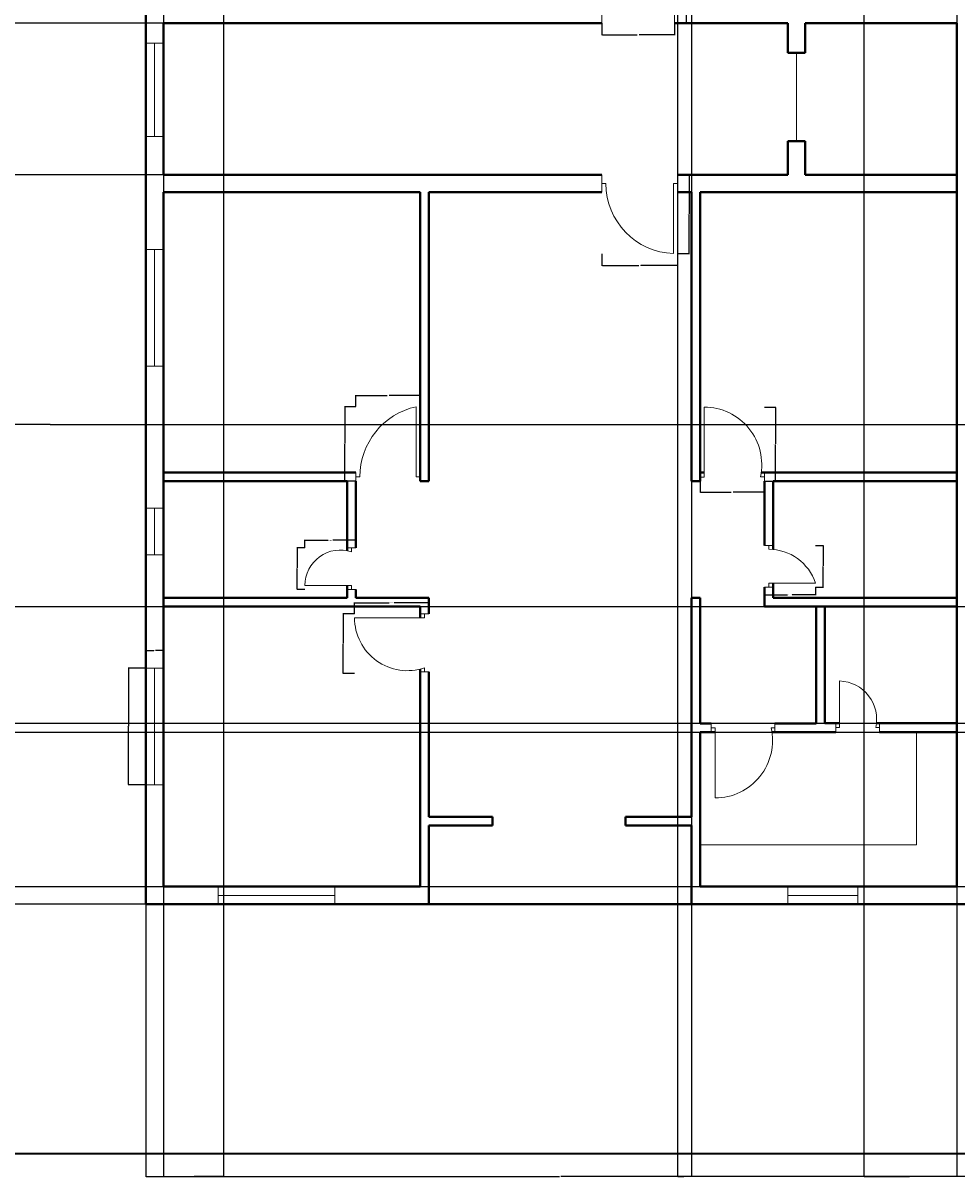
# Model space of a CAD drawing. Units: inches. Extents: x 1355 to 2746, y 1171 to 2751.
# Tile 14 of 24: x 2017 to 2497, y 1171 to 1764. Entities that reach past the tile are written whole.
import ezdxf

# ---------------------------------------------------------------- set-up
doc = ezdxf.new("R2010")
doc.units = ezdxf.units.IN
for name, color, linetype, lineweight in [('A-ANNO-DIMS', 2, 'Continuous', 18), ('A-ANNO-SYMB', 2, 'Continuous', 25), ('A-ANNO-TTLB', 7, 'Continuous', 35), ('A-DOOR', 3, 'Continuous', 20), ('A-FLOR-CASE', 30, 'Continuous', 20), ('A-GLAZ', 4, 'Continuous', 18), ('A-WALL', 7, 'Continuous', 40)]:
    doc.layers.add(name, color=color, linetype=linetype, lineweight=lineweight)
doc.styles.get("Standard").update_dxf_attribs({"font": 'arial.ttf'})
doc.dimstyles.get("Standard").update_dxf_attribs({"dimtxt": 0.18, "dimasz": 0.18, "dimexe": 0.18, "dimexo": 0.0625, "dimgap": 0.09, "dimtad": 0, "dimtih": 1, "dimtoh": 1, "dimdec": 4, "dimzin": 0, "dimdsep": 46, "dimtxsty": 'Standard', "dimcen": 0.09, "dimadec": 0, "dimazin": 0, "dimtfac": 1, "dimtdec": 4, "dimtofl": 0, "dimtmove": 0, "dimatfit": 3, "dimfxl": 1, "dimtolj": 1, "dimtzin": 0, "dimarcsym": 0})

# ---------------------------------------------------------------- blocks, each defined once
blk = doc.blocks.new('WINDOW-PLAN-24')
for p, q in [((0, 24), (9, 24)), ((9, 24), (4.5, 24)), ((4.5, 24), (4.5, 0)), ((4.5, 0), (0, 0)), ((0, 0), (9, 0))]:
    blk.add_line(p, q)
blk = doc.blocks.new('WINDOW-PLAN-60')
for p, q in [((0, 60), (9, 60)), ((9, 60), (4.5, 60)), ((4.5, 60), (4.5, 0)), ((4.5, 0), (0, 0)), ((0, 0), (9, 0))]:
    blk.add_line(p, q)
blk = doc.blocks.new('WINDOW-PLAN-60-2')
for p, q in [((4.5, 60), (0, 60)), ((0, 60), (9, 60)), ((4.5, 0), (4.5, 60)), ((9, 0), (0, 0)), ((0, 0), (4.5, 0))]:
    blk.add_line(p, q)
blk = doc.blocks.new('WINDOW-PLAN-36')
for p, q in [((0, 9), (0, 0)), ((36, 4.5), (36, 9)), ((36, 9), (36, 0)), ((0, 0), (0, 4.5)), ((0, 4.5), (36, 4.5))]:
    blk.add_line(p, q)
blk = doc.blocks.new('WINDOW-PLAN-48')
for p, q in [((9, 48), (0, 48)), ((0, 48), (4.5, 48)), ((4.5, 48), (4.5, 12)), ((4.5, 12), (4.5, 0)), ((4.5, 0), (0, 0)), ((0, 0), (9, 0))]:
    blk.add_line(p, q)
blk = doc.blocks.new('DOOR-ENTRY-N')
for p, q in [((35.29, 4.5), (35.29, 40.5)), ((0, 9), (0, 0)), ((37.29, 9), (37.29, 0)), ((0, 0), (0, 4.5)), ((0, 4.5), (2, 4.5)), ((37.29, 4.5), (35.29, 4.5)), ((37.29, 0), (37.29, 4.5))]:
    blk.add_line(p, q)
blk.add_arc((38.11, 4.5), 36.11, 94.47163, 180)
blk = doc.blocks.new('DOOR-BED-SE')
for p, q in [((2, 2.1), (2, 38.1)), ((0, 2.1), (2, 2.1)), ((33, 2.25), (31, 2.25)), ((33, 0), (33, 4.5)), ((33, 4.5), (33, 2.25))]:
    blk.add_line(p, q)
blk.add_arc((2, 8.44), 29.65, 347.94805, 90)
blk = doc.blocks.new('DOOR-WC-SE')
for p, q in [((0, 21.41), (4.5, 21.41)), ((4.5, 21.41), (2.25, 21.41)), ((2.25, 21.41), (2.25, 19.41)), ((2.25, 0), (2.25, 2)), ((2.25, 2), (26.25, 2)), ((4.5, 0), (0, 0)), ((0, 0), (2.25, 0))]:
    blk.add_line(p, q)
blk.add_arc((2.25, -5.83), 25.25, 18.07862, 90)
blk = doc.blocks.new('DOOR-BED-SW')
for p, q in [((31, 2.25), (31, 38.25)), ((0, 0), (0, 4.5)), ((0, 2.25), (2, 2.25)), ((33, 2.25), (31, 2.25))]:
    blk.add_line(p, q)
blk.add_arc((38.85, 2.25), 36.84, 102.29325, 180)
blk = doc.blocks.new('DOOR-WC-SW')
for p, q in [((21.75, 21.26), (26.25, 21.26)), ((26.25, 21.26), (24, 21.26)), ((24, 21.26), (24, 19.26)), ((24, 2), (0, 2)), ((24, 0), (24, 2)), ((26.25, 0), (21.75, 0)), ((21.75, 0), (24, 0))]:
    blk.add_line(p, q)
blk.add_arc((18.21, 2), 18.21, 71.45684, 180)
blk = doc.blocks.new('DOOR-BEDROOM-SW')
for p, q in [((33.75, 29.78), (38.25, 29.78)), ((38.25, 29.78), (36, 29.78)), ((36, 29.78), (36, 27.78)), ((36, 27.78), (0, 27.78)), ((33.75, 0), (38.25, 0)), ((36, 0), (36, 2)), ((38.25, 0), (36, 0))]:
    blk.add_line(p, q)
blk.add_arc((27.23, 27.78), 27.23, 180, 288.79179)
blk = doc.blocks.new('DOOR-UTILITY-S')
for p, q in [((2, 2.25), (2, 26.25)), ((0, 4.5), (0, 0)), ((0, 0), (0, 2.25)), ((0, 2.25), (2, 2.25)), ((22.55, 2.25), (20.55, 2.25)), ((22.55, 4.5), (22.55, 0)), ((22.55, 0), (22.55, 2.25))]:
    blk.add_line(p, q)
blk.add_arc((1.26, 6.51), 19.76, 347.56133, 87.85632)
blk = doc.blocks.new('DOOR-KITCHEN-S')
for p, q in [((0, 38.25), (0, 33.75)), ((0, 33.75), (0, 36)), ((0, 36), (2, 36)), ((2, 36), (2, 0)), ((32.75, 36), (30.75, 36)), ((32.75, 38.25), (32.75, 33.89)), ((32.75, 33.89), (32.75, 36))]:
    blk.add_line(p, q)
blk.add_arc((2, 29.48), 29.48, 270, 12.78512)
blk = doc.blocks.new('DOOR-ENTRY-S')
for p, q in [((0, 40.5), (0, 31.5)), ((0, 36), (2, 36)), ((38.81, 36), (36.81, 36)), ((36.81, 36), (36.81, 0)), ((38.81, 31.5), (38.81, 40.5))]:
    blk.add_line(p, q)
blk.add_arc((38.02, 36), 36.02, 180, 268.07058)
blk = doc.blocks.new('*D47')
at = {"layer": 'A-ANNO-DIMS', "color": 0, "lineweight": -2, "transparency": 16777216}
for p, q in [((2080.33, 1432.65), (2071.21, 1432.65)), ((2071.39, 1432.47), (2071.39, 1402.84)), ((2071.39, 1372.83), (2071.39, 1402.47)), ((2080.33, 1372.65), (2071.21, 1372.65))]:
    blk.add_line(p, q, dxfattribs=at)
at = {"layer": 'A-ANNO-DIMS', "color": 0, "transparency": 16777216}
for points in [[(2071.36, 1432.47), (2071.42, 1432.47), (2071.39, 1432.65)], [(2071.36, 1372.83), (2071.42, 1372.83), (2071.39, 1372.65)]]:
    blk.add_solid(points, dxfattribs=at)
at = {"layer": 'Defpoints', "color": 0, "transparency": 16777216}
for p in [(2071.39, 1432.65), (2080.39, 1432.65), (2080.39, 1372.65)]:
    blk.add_point(p, dxfattribs=at)
at = {"layer": 'A-ANNO-DIMS', "color": 0, "transparency": 16777216, "insert": (2071.39, 1402.65), "char_height": 0.18, "attachment_point": 5}
blk.add_mtext('\\A1;WINDOW 60 TYP.', dxfattribs=at)
blk = doc.blocks.new('*D48')
at = {"layer": 'A-ANNO-DIMS', "color": 0, "lineweight": -2, "transparency": 16777216}
for p, q in [((2080.39, 1432.72), (2080.39, 1441.83)), ((2080.57, 1441.65), (2084.43, 1441.65)), ((2089.21, 1441.65), (2085.35, 1441.65)), ((2089.39, 1432.72), (2089.39, 1441.83))]:
    blk.add_line(p, q, dxfattribs=at)
at = {"layer": 'A-ANNO-DIMS', "color": 0, "transparency": 16777216}
for points in [[(2080.57, 1441.68), (2080.57, 1441.62), (2080.39, 1441.65)], [(2089.21, 1441.68), (2089.21, 1441.62), (2089.39, 1441.65)]]:
    blk.add_solid(points, dxfattribs=at)
at = {"layer": 'Defpoints', "color": 0, "transparency": 16777216}
for p in [(2089.39, 1441.65), (2080.39, 1432.65), (2089.39, 1432.65)]:
    blk.add_point(p, dxfattribs=at)
at = {"layer": 'A-ANNO-DIMS', "color": 0, "transparency": 16777216, "insert": (2084.89, 1441.65), "char_height": 0.18, "attachment_point": 5}
blk.add_mtext('\\A1;9 TYP.', dxfattribs=at)
blk = doc.blocks.new('*D55')
at = {"layer": 'A-ANNO-DIMS', "color": 0, "lineweight": -2, "transparency": 16777216}
for p, q in [((2352.26, 1804.8), (2358.45, 1804.8)), ((2358.27, 1804.62), (2358.27, 1784.73)), ((2358.27, 1764.48), (2358.27, 1784.37)), ((2352.26, 1764.3), (2358.45, 1764.3))]:
    blk.add_line(p, q, dxfattribs=at)
at = {"layer": 'A-ANNO-DIMS', "color": 0, "transparency": 16777216}
for points in [[(2358.24, 1804.62), (2358.3, 1804.62), (2358.27, 1804.8)], [(2358.24, 1764.48), (2358.3, 1764.48), (2358.27, 1764.3)]]:
    blk.add_solid(points, dxfattribs=at)
at = {"layer": 'Defpoints', "color": 0, "transparency": 16777216}
for p in [(2352.2, 1804.8), (2358.27, 1804.8), (2352.2, 1764.3)]:
    blk.add_point(p, dxfattribs=at)
at = {"layer": 'A-ANNO-DIMS', "color": 0, "transparency": 16777216, "insert": (2358.27, 1784.55), "char_height": 0.18, "attachment_point": 5}
blk.add_mtext('\\A1;ENTRY DOOR 41 TYP.', dxfattribs=at)
blk = doc.blocks.new('*D56')
at = {"layer": 'A-ANNO-DIMS', "color": 0, "lineweight": -2, "transparency": 16777216}
for p, q in [((2314.9, 1764.24), (2314.9, 1758.05)), ((2352.2, 1764.24), (2352.2, 1758.05)), ((2315.08, 1758.23), (2333.02, 1758.23)), ((2352.02, 1758.23), (2334.08, 1758.23))]:
    blk.add_line(p, q, dxfattribs=at)
at = {"layer": 'A-ANNO-DIMS', "color": 0, "transparency": 16777216}
for points in [[(2315.08, 1758.26), (2315.08, 1758.2), (2314.9, 1758.23)], [(2352.02, 1758.26), (2352.02, 1758.2), (2352.2, 1758.23)]]:
    blk.add_solid(points, dxfattribs=at)
at = {"layer": 'Defpoints', "color": 0, "transparency": 16777216}
for p in [(2314.9, 1764.3), (2352.2, 1764.3), (2352.2, 1758.23)]:
    blk.add_point(p, dxfattribs=at)
at = {"layer": 'A-ANNO-DIMS', "color": 0, "transparency": 16777216, "insert": (2333.55, 1758.23), "char_height": 0.18, "attachment_point": 5}
blk.add_mtext('\\A1;37 TYP.', dxfattribs=at)
blk = doc.blocks.new('*D61')
at = {"layer": 'A-ANNO-DIMS', "color": 0, "lineweight": -2, "transparency": 16777216}
for p, q in [((2398.45, 1566.9), (2404.29, 1566.9)), ((2404.11, 1566.72), (2404.11, 1548.03)), ((2404.11, 1528.98), (2404.11, 1547.67)), ((2398.45, 1528.8), (2404.29, 1528.8))]:
    blk.add_line(p, q, dxfattribs=at)
at = {"layer": 'A-ANNO-DIMS', "color": 0, "transparency": 16777216}
for points in [[(2404.08, 1566.72), (2404.14, 1566.72), (2404.11, 1566.9)], [(2404.08, 1528.98), (2404.14, 1528.98), (2404.11, 1528.8)]]:
    blk.add_solid(points, dxfattribs=at)
at = {"layer": 'Defpoints', "color": 0, "transparency": 16777216}
for p in [(2398.39, 1566.9), (2404.11, 1566.9), (2398.39, 1528.8)]:
    blk.add_point(p, dxfattribs=at)
at = {"layer": 'A-ANNO-DIMS', "color": 0, "transparency": 16777216, "insert": (2404.11, 1547.85), "char_height": 0.18, "attachment_point": 5}
blk.add_mtext('\\A1;BED DOOR 38 TYP.', dxfattribs=at)
blk = doc.blocks.new('*D62')
at = {"layer": 'A-ANNO-DIMS', "color": 0, "lineweight": -2, "transparency": 16777216}
for p, q in [((2365.39, 1528.74), (2365.39, 1522.91)), ((2398.39, 1528.74), (2398.39, 1522.91)), ((2365.57, 1523.09), (2381.36, 1523.09)), ((2398.21, 1523.09), (2382.42, 1523.09))]:
    blk.add_line(p, q, dxfattribs=at)
at = {"layer": 'A-ANNO-DIMS', "color": 0, "transparency": 16777216}
for points in [[(2365.57, 1523.12), (2365.57, 1523.06), (2365.39, 1523.09)], [(2398.21, 1523.12), (2398.21, 1523.06), (2398.39, 1523.09)]]:
    blk.add_solid(points, dxfattribs=at)
at = {"layer": 'Defpoints', "color": 0, "transparency": 16777216}
for p in [(2365.39, 1528.8), (2398.39, 1528.8), (2398.39, 1523.09)]:
    blk.add_point(p, dxfattribs=at)
at = {"layer": 'A-ANNO-DIMS', "color": 0, "transparency": 16777216, "insert": (2381.89, 1523.09), "char_height": 0.18, "attachment_point": 5}
blk.add_mtext('\\A1;33 TYP.', dxfattribs=at)
blk = doc.blocks.new('*D63')
at = {"layer": 'A-ANNO-DIMS', "color": 0, "lineweight": -2, "transparency": 16777216}
for p, q in [((2398.39, 1474.28), (2398.39, 1470.22)), ((2424.64, 1474.28), (2424.64, 1470.22)), ((2398.57, 1470.4), (2410.33, 1470.4)), ((2424.46, 1470.4), (2412.7, 1470.4))]:
    blk.add_line(p, q, dxfattribs=at)
at = {"layer": 'A-ANNO-DIMS', "color": 0, "transparency": 16777216}
for points in [[(2398.57, 1470.43), (2398.57, 1470.37), (2398.39, 1470.4)], [(2424.46, 1470.43), (2424.46, 1470.37), (2424.64, 1470.4)]]:
    blk.add_solid(points, dxfattribs=at)
at = {"layer": 'Defpoints', "color": 0, "transparency": 16777216}
for p in [(2398.39, 1474.34), (2424.64, 1474.34), (2424.64, 1470.4)]:
    blk.add_point(p, dxfattribs=at)
at = {"layer": 'A-ANNO-DIMS', "color": 0, "transparency": 16777216, "insert": (2411.52, 1470.4), "char_height": 0.18, "attachment_point": 5}
blk.add_mtext('\\A1;WC DOOR 26 TYP.', dxfattribs=at)
blk = doc.blocks.new('*D64')
at = {"layer": 'A-ANNO-DIMS', "color": 0, "lineweight": -2, "transparency": 16777216}
for p, q in [((2424.7, 1495.75), (2428.76, 1495.75)), ((2428.58, 1495.57), (2428.58, 1485.23)), ((2428.58, 1474.52), (2428.58, 1484.87)), ((2424.7, 1474.34), (2428.76, 1474.34))]:
    blk.add_line(p, q, dxfattribs=at)
at = {"layer": 'A-ANNO-DIMS', "color": 0, "transparency": 16777216}
for points in [[(2428.55, 1495.57), (2428.61, 1495.57), (2428.58, 1495.75)], [(2428.55, 1474.52), (2428.61, 1474.52), (2428.58, 1474.34)]]:
    blk.add_solid(points, dxfattribs=at)
at = {"layer": 'Defpoints', "color": 0, "transparency": 16777216}
for p in [(2424.64, 1495.75), (2428.58, 1495.75), (2424.64, 1474.34)]:
    blk.add_point(p, dxfattribs=at)
at = {"layer": 'A-ANNO-DIMS', "color": 0, "transparency": 16777216, "insert": (2428.58, 1485.05), "char_height": 0.18, "attachment_point": 5}
blk.add_mtext('\\A1;21 TYP.', dxfattribs=at)
blk = doc.blocks.new('*D65')
at = {"layer": 'A-ANNO-DIMS', "color": 0, "lineweight": -2, "transparency": 16777216}
for p, q in [((2188.33, 1567.05), (2182.47, 1567.05)), ((2182.65, 1566.87), (2182.65, 1548.11)), ((2182.65, 1528.98), (2182.65, 1547.74)), ((2188.33, 1528.8), (2182.47, 1528.8))]:
    blk.add_line(p, q, dxfattribs=at)
at = {"layer": 'A-ANNO-DIMS', "color": 0, "transparency": 16777216}
for points in [[(2182.62, 1566.87), (2182.68, 1566.87), (2182.65, 1567.05)], [(2182.62, 1528.98), (2182.68, 1528.98), (2182.65, 1528.8)]]:
    blk.add_solid(points, dxfattribs=at)
at = {"layer": 'Defpoints', "color": 0, "transparency": 16777216}
for p in [(2182.65, 1567.05), (2188.39, 1567.05), (2188.39, 1528.8)]:
    blk.add_point(p, dxfattribs=at)
at = {"layer": 'A-ANNO-DIMS', "color": 0, "transparency": 16777216, "insert": (2182.65, 1547.93), "char_height": 0.18, "attachment_point": 5}
blk.add_mtext('\\A1;BED DOOR 38 TYP.', dxfattribs=at)
blk = doc.blocks.new('*D66')
at = {"layer": 'A-ANNO-DIMS', "color": 0, "lineweight": -2, "transparency": 16777216}
for p, q in [((2188.39, 1567.11), (2188.39, 1572.97)), ((2188.57, 1572.79), (2204.36, 1572.79)), ((2221.21, 1572.79), (2205.42, 1572.79)), ((2221.39, 1567.11), (2221.39, 1572.97))]:
    blk.add_line(p, q, dxfattribs=at)
at = {"layer": 'A-ANNO-DIMS', "color": 0, "transparency": 16777216}
for points in [[(2188.57, 1572.82), (2188.57, 1572.76), (2188.39, 1572.79)], [(2221.21, 1572.82), (2221.21, 1572.76), (2221.39, 1572.79)]]:
    blk.add_solid(points, dxfattribs=at)
at = {"layer": 'Defpoints', "color": 0, "transparency": 16777216}
for p in [(2221.39, 1572.79), (2188.39, 1567.05), (2221.39, 1567.05)]:
    blk.add_point(p, dxfattribs=at)
at = {"layer": 'A-ANNO-DIMS', "color": 0, "transparency": 16777216, "insert": (2204.89, 1572.79), "char_height": 0.18, "attachment_point": 5}
blk.add_mtext('\\A1;33 TYP.', dxfattribs=at)
blk = doc.blocks.new('*D67')
at = {"layer": 'A-ANNO-DIMS', "color": 0, "lineweight": -2, "transparency": 16777216}
for p, q in [((2162.14, 1494.48), (2162.14, 1498.54)), ((2162.32, 1498.36), (2174.08, 1498.36)), ((2188.21, 1498.36), (2176.45, 1498.36)), ((2188.39, 1494.48), (2188.39, 1498.54))]:
    blk.add_line(p, q, dxfattribs=at)
at = {"layer": 'A-ANNO-DIMS', "color": 0, "transparency": 16777216}
for points in [[(2162.32, 1498.39), (2162.32, 1498.33), (2162.14, 1498.36)], [(2188.21, 1498.39), (2188.21, 1498.33), (2188.39, 1498.36)]]:
    blk.add_solid(points, dxfattribs=at)
at = {"layer": 'Defpoints', "color": 0, "transparency": 16777216}
for p in [(2188.39, 1498.36), (2162.14, 1494.42), (2188.39, 1494.42)]:
    blk.add_point(p, dxfattribs=at)
at = {"layer": 'A-ANNO-DIMS', "color": 0, "transparency": 16777216, "insert": (2175.27, 1498.36), "char_height": 0.18, "attachment_point": 5}
blk.add_mtext('\\A1;WC DOOR 26 TYP.', dxfattribs=at)
blk = doc.blocks.new('*D68')
at = {"layer": 'A-ANNO-DIMS', "color": 0, "lineweight": -2, "transparency": 16777216}
for p, q in [((2162.08, 1494.42), (2158.02, 1494.42)), ((2158.2, 1494.24), (2158.2, 1483.97)), ((2158.2, 1473.34), (2158.2, 1483.61)), ((2162.08, 1473.16), (2158.02, 1473.16))]:
    blk.add_line(p, q, dxfattribs=at)
at = {"layer": 'A-ANNO-DIMS', "color": 0, "transparency": 16777216}
for points in [[(2158.17, 1494.24), (2158.23, 1494.24), (2158.2, 1494.42)], [(2158.17, 1473.34), (2158.23, 1473.34), (2158.2, 1473.16)]]:
    blk.add_solid(points, dxfattribs=at)
at = {"layer": 'Defpoints', "color": 0, "transparency": 16777216}
for p in [(2158.2, 1494.42), (2162.14, 1494.42), (2162.14, 1473.16)]:
    blk.add_point(p, dxfattribs=at)
at = {"layer": 'A-ANNO-DIMS', "color": 0, "transparency": 16777216, "insert": (2158.2, 1483.79), "char_height": 0.18, "attachment_point": 5}
blk.add_mtext('\\A1;21 TYP.', dxfattribs=at)
blk = doc.blocks.new('*D69')
at = {"layer": 'A-ANNO-DIMS', "color": 0, "lineweight": -2, "transparency": 16777216}
for p, q in [((2187.64, 1460.63), (2187.64, 1466.48)), ((2187.82, 1466.3), (2205.54, 1466.3)), ((2225.71, 1466.3), (2208, 1466.3)), ((2225.89, 1460.63), (2225.89, 1466.48))]:
    blk.add_line(p, q, dxfattribs=at)
at = {"layer": 'A-ANNO-DIMS', "color": 0, "transparency": 16777216}
for points in [[(2187.82, 1466.33), (2187.82, 1466.27), (2187.64, 1466.3)], [(2225.71, 1466.33), (2225.71, 1466.27), (2225.89, 1466.3)]]:
    blk.add_solid(points, dxfattribs=at)
at = {"layer": 'Defpoints', "color": 0, "transparency": 16777216}
for p in [(2225.89, 1466.3), (2187.64, 1460.56), (2225.89, 1460.56)]:
    blk.add_point(p, dxfattribs=at)
at = {"layer": 'A-ANNO-DIMS', "color": 0, "transparency": 16777216, "insert": (2206.77, 1466.3), "char_height": 0.18, "attachment_point": 5}
blk.add_mtext('\\A1;BED DOOR 38 TYP.', dxfattribs=at)
blk = doc.blocks.new('*D70')
at = {"layer": 'A-ANNO-DIMS', "color": 0, "lineweight": -2, "transparency": 16777216}
for p, q in [((2187.58, 1460.56), (2181.72, 1460.56)), ((2181.9, 1460.38), (2181.9, 1445.44)), ((2181.9, 1430.14), (2181.9, 1445.08)), ((2187.58, 1429.96), (2181.72, 1429.96))]:
    blk.add_line(p, q, dxfattribs=at)
at = {"layer": 'A-ANNO-DIMS', "color": 0, "transparency": 16777216}
for points in [[(2181.87, 1460.38), (2181.93, 1460.38), (2181.9, 1460.56)], [(2181.87, 1430.14), (2181.93, 1430.14), (2181.9, 1429.96)]]:
    blk.add_solid(points, dxfattribs=at)
at = {"layer": 'Defpoints', "color": 0, "transparency": 16777216}
for p in [(2181.9, 1460.56), (2187.64, 1460.56), (2187.64, 1429.96)]:
    blk.add_point(p, dxfattribs=at)
at = {"layer": 'A-ANNO-DIMS', "color": 0, "transparency": 16777216, "insert": (2181.9, 1445.26), "char_height": 0.18, "attachment_point": 5}
blk.add_mtext('\\A1;31 TYP.', dxfattribs=at)
blk = doc.blocks.new('*D83')
at = {"layer": 'A-ANNO-DIMS', "color": 0, "lineweight": -2, "transparency": 16777216}
for p, q in [((2353.77, 1686.3), (2359.97, 1686.3)), ((2359.79, 1686.12), (2359.79, 1666.23)), ((2359.79, 1645.98), (2359.79, 1665.87)), ((2353.77, 1645.8), (2359.97, 1645.8))]:
    blk.add_line(p, q, dxfattribs=at)
at = {"layer": 'A-ANNO-DIMS', "color": 0, "transparency": 16777216}
for points in [[(2359.76, 1686.12), (2359.82, 1686.12), (2359.79, 1686.3)], [(2359.76, 1645.98), (2359.82, 1645.98), (2359.79, 1645.8)]]:
    blk.add_solid(points, dxfattribs=at)
at = {"layer": 'Defpoints', "color": 0, "transparency": 16777216}
for p in [(2353.71, 1686.3), (2359.79, 1686.3), (2353.71, 1645.8)]:
    blk.add_point(p, dxfattribs=at)
at = {"layer": 'A-ANNO-DIMS', "color": 0, "transparency": 16777216, "insert": (2359.79, 1666.05), "char_height": 0.18, "attachment_point": 5}
blk.add_mtext('\\A1;ENTRY DOOR 41 TYP.', dxfattribs=at)
blk = doc.blocks.new('*D84')
at = {"layer": 'A-ANNO-DIMS', "color": 0, "lineweight": -2, "transparency": 16777216}
for p, q in [((2314.9, 1645.74), (2314.9, 1639.55)), ((2353.71, 1645.74), (2353.71, 1639.55)), ((2315.08, 1639.73), (2333.78, 1639.73)), ((2353.53, 1639.73), (2334.83, 1639.73))]:
    blk.add_line(p, q, dxfattribs=at)
at = {"layer": 'A-ANNO-DIMS', "color": 0, "transparency": 16777216}
for points in [[(2315.08, 1639.76), (2315.08, 1639.7), (2314.9, 1639.73)], [(2353.53, 1639.76), (2353.53, 1639.7), (2353.71, 1639.73)]]:
    blk.add_solid(points, dxfattribs=at)
at = {"layer": 'Defpoints', "color": 0, "transparency": 16777216}
for p in [(2314.9, 1645.8), (2353.71, 1645.8), (2353.71, 1639.73)]:
    blk.add_point(p, dxfattribs=at)
at = {"layer": 'A-ANNO-DIMS', "color": 0, "transparency": 16777216, "insert": (2334.31, 1639.73), "char_height": 0.18, "attachment_point": 5}
blk.add_mtext('\\A1;39 TYP.', dxfattribs=at)
blk = doc.blocks.new('*D97')
at = {"layer": 'A-ANNO-DIMS', "color": 0, "lineweight": -2, "transparency": 16777216}
for p, q in [((2080.39, 1311.24), (2080.39, 1171.06)), ((2506.39, 1311.24), (2506.39, 1171.06)), ((2080.57, 1171.24), (2293.1, 1171.24)), ((2506.21, 1171.24), (2293.68, 1171.24))]:
    blk.add_line(p, q, dxfattribs=at)
at = {"layer": 'A-ANNO-DIMS', "color": 0, "transparency": 16777216}
for points in [[(2080.57, 1171.27), (2080.57, 1171.21), (2080.39, 1171.24)], [(2506.21, 1171.27), (2506.21, 1171.21), (2506.39, 1171.24)]]:
    blk.add_solid(points, dxfattribs=at)
at = {"layer": 'Defpoints', "color": 0, "transparency": 16777216}
for p in [(2080.39, 1311.3), (2506.39, 1311.3), (2506.39, 1171.24)]:
    blk.add_point(p, dxfattribs=at)
at = {"layer": 'A-ANNO-DIMS', "color": 0, "transparency": 16777216, "insert": (2293.39, 1171.24), "char_height": 0.18, "attachment_point": 5}
blk.add_mtext('\\A1;426', dxfattribs=at)
blk = doc.blocks.new('*D102')
at = {"layer": 'A-ANNO-DIMS', "color": 0, "lineweight": -2, "transparency": 16777216}
for p, q in [((2089.33, 1764.3), (1407.53, 1764.3)), ((1407.71, 1764.12), (1407.71, 1725.48)), ((1407.71, 1686.48), (1407.71, 1725.12)), ((2089.33, 1686.3), (1407.53, 1686.3))]:
    blk.add_line(p, q, dxfattribs=at)
at = {"layer": 'A-ANNO-DIMS', "color": 0, "transparency": 16777216}
for points in [[(1407.68, 1764.12), (1407.74, 1764.12), (1407.71, 1764.3)], [(1407.68, 1686.48), (1407.74, 1686.48), (1407.71, 1686.3)]]:
    blk.add_solid(points, dxfattribs=at)
at = {"layer": 'Defpoints', "color": 0, "transparency": 16777216}
for p in [(1407.71, 1764.3), (2089.39, 1764.3), (2089.39, 1686.3)]:
    blk.add_point(p, dxfattribs=at)
at = {"layer": 'A-ANNO-DIMS', "color": 0, "transparency": 16777216, "insert": (1407.71, 1725.3), "char_height": 0.18, "attachment_point": 5}
blk.add_mtext('\\A1;78', dxfattribs=at)
blk = doc.blocks.new('*D106')
at = {"layer": 'A-ANNO-DIMS', "color": 0, "lineweight": -2, "transparency": 16777216}
for p, q in [((2031.09, 1557.85), (1407.53, 1557.85)), ((1407.71, 1557.67), (1407.71, 1434.76)), ((1407.71, 1311.48), (1407.71, 1434.39)), ((2080.33, 1311.3), (1407.53, 1311.3))]:
    blk.add_line(p, q, dxfattribs=at)
at = {"layer": 'A-ANNO-DIMS', "color": 0, "transparency": 16777216}
for points in [[(1407.68, 1557.67), (1407.74, 1557.67), (1407.71, 1557.85)], [(1407.68, 1311.48), (1407.74, 1311.48), (1407.71, 1311.3)]]:
    blk.add_solid(points, dxfattribs=at)
at = {"layer": 'Defpoints', "color": 0, "transparency": 16777216}
for p in [(1407.71, 1557.85), (2031.15, 1557.85), (2080.39, 1311.3)]:
    blk.add_point(p, dxfattribs=at)
at = {"layer": 'A-ANNO-DIMS', "color": 0, "transparency": 16777216, "insert": (1407.71, 1434.57), "char_height": 0.18, "attachment_point": 5}
blk.add_mtext('\\A1;246.54', dxfattribs=at)
blk = doc.blocks.new('*D107')
at = {"layer": 'A-ANNO-DIMS', "color": 0, "lineweight": -2, "transparency": 16777216}
for p, q in [((2089.33, 1686.3), (1407.53, 1686.3)), ((1407.71, 1686.12), (1407.71, 1622.26)), ((1407.71, 1558.03), (1407.71, 1621.89)), ((2031.09, 1557.85), (1407.53, 1557.85))]:
    blk.add_line(p, q, dxfattribs=at)
at = {"layer": 'A-ANNO-DIMS', "color": 0, "transparency": 16777216}
for points in [[(1407.68, 1686.12), (1407.74, 1686.12), (1407.71, 1686.3)], [(1407.68, 1558.03), (1407.74, 1558.03), (1407.71, 1557.85)]]:
    blk.add_solid(points, dxfattribs=at)
at = {"layer": 'Defpoints', "color": 0, "transparency": 16777216}
for p in [(1407.71, 1686.3), (2089.39, 1686.3), (2031.15, 1557.85)]:
    blk.add_point(p, dxfattribs=at)
at = {"layer": 'A-ANNO-DIMS', "color": 0, "transparency": 16777216, "insert": (1407.71, 1622.07), "char_height": 0.18, "attachment_point": 5}
blk.add_mtext('\\A1;128.46', dxfattribs=at)
blk = doc.blocks.new('*D108')
at = {"layer": 'A-ANNO-DIMS', "color": 0, "lineweight": -2, "transparency": 16777216}
for p, q in [((2089.39, 2130.24), (2089.39, 1171.06)), ((2120.28, 2130.24), (2120.28, 1171.06)), ((2089.57, 1171.24), (2104.44, 1171.24)), ((2120.1, 1171.24), (2105.23, 1171.24))]:
    blk.add_line(p, q, dxfattribs=at)
at = {"layer": 'A-ANNO-DIMS', "color": 0, "transparency": 16777216}
for points in [[(2089.57, 1171.27), (2089.57, 1171.21), (2089.39, 1171.24)], [(2120.1, 1171.27), (2120.1, 1171.21), (2120.28, 1171.24)]]:
    blk.add_solid(points, dxfattribs=at)
at = {"layer": 'Defpoints', "color": 0, "transparency": 16777216}
for p in [(2089.39, 2130.3), (2120.28, 2130.3), (2120.28, 1171.24)]:
    blk.add_point(p, dxfattribs=at)
at = {"layer": 'A-ANNO-DIMS', "color": 0, "transparency": 16777216, "insert": (2104.84, 1171.24), "char_height": 0.18, "attachment_point": 5}
blk.add_mtext('\\A1;30.89', dxfattribs=at)
blk = doc.blocks.new('*D109')
at = {"layer": 'A-ANNO-DIMS', "color": 0, "lineweight": -2, "transparency": 16777216}
for p, q in [((2449.47, 2130.24), (2449.47, 1171.06)), ((2497.39, 2130.24), (2497.39, 1171.06)), ((2449.65, 1171.24), (2473.04, 1171.24)), ((2497.21, 1171.24), (2473.83, 1171.24))]:
    blk.add_line(p, q, dxfattribs=at)
at = {"layer": 'A-ANNO-DIMS', "color": 0, "transparency": 16777216}
for points in [[(2449.65, 1171.27), (2449.65, 1171.21), (2449.47, 1171.24)], [(2497.21, 1171.27), (2497.21, 1171.21), (2497.39, 1171.24)]]:
    blk.add_solid(points, dxfattribs=at)
at = {"layer": 'Defpoints', "color": 0, "transparency": 16777216}
for p in [(2449.47, 2130.3), (2497.39, 2130.3), (2497.39, 1171.24)]:
    blk.add_point(p, dxfattribs=at)
at = {"layer": 'A-ANNO-DIMS', "color": 0, "transparency": 16777216, "insert": (2473.43, 1171.24), "char_height": 0.18, "attachment_point": 5}
blk.add_mtext('\\A1;47.92', dxfattribs=at)
blk = doc.blocks.new('*D126')
at = {"layer": 'A-ANNO-DIMS', "color": 0, "lineweight": -2, "transparency": 16777216}
for p, q in [((2080.39, 2219.34), (2080.39, 1171.06)), ((2506.39, 2219.34), (2506.39, 1171.06)), ((2080.57, 1171.24), (2293.1, 1171.24)), ((2506.21, 1171.24), (2293.68, 1171.24))]:
    blk.add_line(p, q, dxfattribs=at)
at = {"layer": 'A-ANNO-DIMS', "color": 0, "transparency": 16777216}
for points in [[(2080.57, 1171.27), (2080.57, 1171.21), (2080.39, 1171.24)], [(2506.21, 1171.27), (2506.21, 1171.21), (2506.39, 1171.24)]]:
    blk.add_solid(points, dxfattribs=at)
at = {"layer": 'Defpoints', "color": 0, "transparency": 16777216}
for p in [(2080.39, 2219.4), (2506.39, 2219.4), (2506.39, 1171.24)]:
    blk.add_point(p, dxfattribs=at)
at = {"layer": 'A-ANNO-DIMS', "color": 0, "transparency": 16777216, "insert": (2293.39, 1171.24), "char_height": 0.18, "attachment_point": 5}
blk.add_mtext('\\A1;426', dxfattribs=at)
blk = doc.blocks.new('*D134')
at = {"layer": 'A-ANNO-DIMS', "color": 0, "lineweight": -2, "transparency": 16777216}
for p, q in [((2353.71, 2477.34), (2353.71, 1171.06)), ((2360.89, 2477.34), (2360.89, 1171.06)), ((2353.89, 1171.24), (2356.92, 1171.24)), ((2360.71, 1171.24), (2357.68, 1171.24))]:
    blk.add_line(p, q, dxfattribs=at)
at = {"layer": 'A-ANNO-DIMS', "color": 0, "transparency": 16777216}
for points in [[(2353.89, 1171.27), (2353.89, 1171.21), (2353.71, 1171.24)], [(2360.71, 1171.27), (2360.71, 1171.21), (2360.89, 1171.24)]]:
    blk.add_solid(points, dxfattribs=at)
at = {"layer": 'Defpoints', "color": 0, "transparency": 16777216}
for p in [(2353.71, 2477.4), (2360.89, 2477.4), (2360.89, 1171.24)]:
    blk.add_point(p, dxfattribs=at)
at = {"layer": 'A-ANNO-DIMS', "color": 0, "transparency": 16777216, "insert": (2357.3, 1171.24), "char_height": 0.18, "attachment_point": 5}
blk.add_mtext('\\A1;7.181', dxfattribs=at)
blk = doc.blocks.new('*D142')
at = {"layer": 'A-ANNO-DIMS', "color": 0, "lineweight": -2, "transparency": 16777216}
for p, q in [((1931.77, 1399.8), (2648.07, 1399.8)), ((2647.89, 1399.62), (2647.89, 1360.23)), ((2647.89, 1320.48), (2647.89, 1359.87)), ((1931.77, 1320.3), (2648.07, 1320.3))]:
    blk.add_line(p, q, dxfattribs=at)
at = {"layer": 'A-ANNO-DIMS', "color": 0, "transparency": 16777216}
for points in [[(2647.86, 1399.62), (2647.92, 1399.62), (2647.89, 1399.8)], [(2647.86, 1320.48), (2647.92, 1320.48), (2647.89, 1320.3)]]:
    blk.add_solid(points, dxfattribs=at)
at = {"layer": 'Defpoints', "color": 0, "transparency": 16777216}
for p in [(1931.71, 1399.8), (2647.89, 1399.8), (1931.71, 1320.3)]:
    blk.add_point(p, dxfattribs=at)
at = {"layer": 'A-ANNO-DIMS', "color": 0, "transparency": 16777216, "insert": (2647.89, 1360.05), "char_height": 0.18, "attachment_point": 5}
blk.add_mtext('\\A1;79.5', dxfattribs=at)
blk = doc.blocks.new('*D143')
at = {"layer": 'A-ANNO-DIMS', "color": 0, "lineweight": -2, "transparency": 16777216}
for p, q in [((1931.77, 1464.3), (2648.07, 1464.3)), ((2647.89, 1464.12), (2647.89, 1434.48)), ((2647.89, 1404.48), (2647.89, 1434.12)), ((1931.77, 1404.3), (2648.07, 1404.3))]:
    blk.add_line(p, q, dxfattribs=at)
at = {"layer": 'A-ANNO-DIMS', "color": 0, "transparency": 16777216}
for points in [[(2647.86, 1464.12), (2647.92, 1464.12), (2647.89, 1464.3)], [(2647.86, 1404.48), (2647.92, 1404.48), (2647.89, 1404.3)]]:
    blk.add_solid(points, dxfattribs=at)
at = {"layer": 'Defpoints', "color": 0, "transparency": 16777216}
for p in [(1931.71, 1464.3), (2647.89, 1464.3), (1931.71, 1404.3)]:
    blk.add_point(p, dxfattribs=at)
at = {"layer": 'A-ANNO-DIMS', "color": 0, "transparency": 16777216, "insert": (2647.89, 1434.3), "char_height": 0.18, "attachment_point": 5}
blk.add_mtext('\\A1;60', dxfattribs=at)

msp = doc.modelspace()

# ---------------------------------------------------------------- linework, layer by layer
at = {"layer": 'A-ANNO-SYMB'}
msp.add_line((2031.1535, 1557.845), (2576.886, 1557.845), dxfattribs=at)
at = {"layer": 'A-ANNO-TTLB'}
msp.add_lwpolyline([(1355.0901, 2751.4741), (2746.1804, 2751.4741), (2746.1804, 1182.883), (1355.0901, 1182.883)], close=True, dxfattribs=at)
at = {"layer": 'A-DOOR'}
msp.add_line((2414.8909, 1748.9343), (2414.8909, 1703.5696), dxfattribs=at)
at = {"layer": 'A-FLOR-CASE'}
for p, q in [((2476.5667, 1341.7851), (2476.5667, 1399.8018)), ((2365.3909, 1341.7851), (2476.5667, 1341.7851))]:
    msp.add_line(p, q, dxfattribs=at)
at = {"layer": 'A-WALL'}
for p, q in [((2080.3909, 2139.3018), (2080.3909, 1311.3018)), ((2089.3909, 1764.3018), (2221.3909, 1764.3018)), ((2089.3909, 1764.3018), (2089.3909, 1686.3018)), ((2221.3909, 1764.3018), (2314.9023, 1764.3018)), ((2352.1969, 1764.3018), (2410.3909, 1764.3018)), ((2410.3909, 1764.3018), (2410.3909, 1748.9343)), ((2419.3909, 1764.3018), (2497.3909, 1764.3018)), ((2419.3909, 1764.3018), (2419.3909, 1748.9343)), ((2497.3909, 1764.3018), (2497.3909, 1320.3018)), ((2410.3909, 1748.9343), (2419.3909, 1748.9343)), ((2410.3909, 1703.5696), (2410.3909, 1686.3018)), ((2410.3909, 1703.5696), (2419.3909, 1703.5696)), ((2419.3909, 1703.5696), (2419.3909, 1686.3018)), ((2298.3718, 1686.3018), (2089.3909, 1686.3018)), ((2298.3718, 1686.3018), (2314.9023, 1686.3018)), ((2410.3909, 1686.3018), (2353.71, 1686.3018)), ((2419.3909, 1686.3018), (2497.3909, 1686.3018)), ((2089.3909, 1677.3018), (2089.3909, 1320.3018)), ((2221.3909, 1677.3018), (2089.3909, 1677.3018)), ((2221.3909, 1677.3018), (2221.3909, 1528.8018)), ((2225.8909, 1677.3018), (2225.8909, 1528.8018)), ((2298.3718, 1677.3018), (2225.8909, 1677.3018)), ((2314.9023, 1677.3018), (2298.3718, 1677.3018)), ((2360.8909, 1677.3018), (2353.71, 1677.3018)), ((2360.8909, 1677.3018), (2360.8909, 1528.8018)), ((2365.3909, 1677.3018), (2365.3909, 1528.8018)), ((2410.3909, 1677.3018), (2365.3909, 1677.3018)), ((2410.3909, 1677.3018), (2497.3909, 1677.3018)), ((2188.3909, 1533.3018), (2089.3909, 1533.3018)), ((2367.3909, 1533.3018), (2365.3909, 1533.3018)), ((2410.3909, 1533.3018), (2396.7813, 1533.3018)), ((2410.3909, 1533.3018), (2497.3909, 1533.3018)), ((2183.8909, 1528.8018), (2089.3909, 1528.8018)), ((2089.3909, 1528.8018), (2183.8909, 1528.8018)), ((2183.8909, 1528.8018), (2183.8909, 1493.0182)), ((2188.3909, 1528.8018), (2188.3909, 1494.4205)), ((2225.8909, 1528.8018), (2221.3909, 1528.8018)), ((2365.3909, 1528.8018), (2360.8909, 1528.8018)), ((2398.3909, 1528.8018), (2398.3909, 1495.7519)), ((2410.3909, 1528.8018), (2402.8909, 1528.8018)), ((2497.3909, 1528.8018), (2402.8909, 1528.8018)), ((2402.8909, 1528.8018), (2402.8909, 1493.6514)), ((2410.3909, 1528.8018), (2497.3909, 1528.8018)), ((2183.8909, 1475.1566), (2183.8909, 1468.8018)), ((2188.3909, 1473.1566), (2188.3909, 1468.8018)), ((2398.3909, 1474.34), (2398.3909, 1468.8018)), ((2402.8909, 1476.34), (2402.8909, 1468.8018)), ((2183.8909, 1468.8018), (2089.3909, 1468.8018)), ((2225.8909, 1468.8018), (2188.3909, 1468.8018)), ((2188.3909, 1468.8018), (2192.8909, 1468.8018)), ((2225.8909, 1468.8018), (2225.8909, 1460.5634)), ((2360.8909, 1468.8018), (2360.8909, 1356.2098)), ((2365.3909, 1468.8018), (2360.8909, 1468.8018)), ((2365.3909, 1464.3018), (2365.3909, 1468.8018)), ((2398.3909, 1464.3018), (2398.3909, 1468.8018)), ((2410.3909, 1468.8018), (2402.8909, 1468.8018)), ((2410.3909, 1468.8018), (2497.3909, 1468.8018)), ((2221.3909, 1464.3018), (2089.3909, 1464.3018)), ((2221.3909, 1464.3018), (2221.3909, 1458.5634)), ((2365.3909, 1464.3018), (2365.3909, 1404.1662)), ((2410.3909, 1464.3018), (2398.3909, 1464.3018)), ((2410.3909, 1464.3018), (2497.3909, 1464.3018)), ((2425.0397, 1404.1662), (2425.0397, 1464.3018)), ((2425.0397, 1464.3018), (2429.5397, 1464.3018)), ((2429.5397, 1464.3018), (2429.5397, 1404.3018)), ((2497.3909, 1464.3018), (2497.3909, 1399.8018)), ((2221.3909, 1432.127), (2221.3909, 1320.3018)), ((2225.8909, 1430.786), (2225.8909, 1356.2098)), ((2371.0907, 1404.1662), (2365.3909, 1404.1662)), ((2425.0397, 1404.1662), (2403.8368, 1404.1662)), ((2429.5397, 1404.3018), (2437.1011, 1404.3018)), ((2456.018, 1404.3018), (2497.3909, 1404.3018)), ((2365.3909, 1399.6662), (2365.3909, 1320.3018)), ((2365.3909, 1399.6662), (2373.0907, 1399.6662)), ((2403.8368, 1399.8018), (2402.2361, 1399.802)), ((2435.1011, 1399.8018), (2403.8368, 1399.8018)), ((2497.3909, 1399.8018), (2457.6563, 1399.8018)), ((2258.6044, 1356.2098), (2225.8909, 1356.2098)), ((2258.6044, 1356.2098), (2258.6044, 1351.7098)), ((2360.8909, 1356.2098), (2326.9423, 1356.2098)), ((2326.9423, 1356.2098), (2326.9423, 1351.7098)), ((2225.8909, 1351.7098), (2225.8909, 1320.3018)), ((2225.8909, 1351.7098), (2258.6044, 1351.7098)), ((2225.8909, 1351.7098), (2225.8909, 1311.3018)), ((2326.9423, 1351.7098), (2360.8909, 1351.7098)), ((2360.8909, 1351.7098), (2360.8909, 1320.3018)), ((2221.3909, 1320.3018), (2089.3909, 1320.3018)), ((2360.8909, 1320.3018), (2360.8909, 1311.3018)), ((2497.3909, 1320.3018), (2365.3909, 1320.3018)), ((2410.3909, 1320.3018), (2497.3909, 1320.3018)), ((2225.8909, 1311.3018), (2080.3909, 1311.3018)), ((2225.8909, 1311.3018), (2360.8909, 1311.3018)), ((2506.3909, 1311.3018), (2360.8909, 1311.3018)), ((2410.3909, 1311.3018), (2497.3909, 1311.3018))]:
    msp.add_line(p, q, dxfattribs=at)

# ---------------------------------------------------------------- block references
at = {"layer": 'A-DOOR'}
for name, p in [('DOOR-ENTRY-N', (2314.9026, 1764.302)), ('DOOR-ENTRY-S', (2314.9026, 1645.802)), ('DOOR-BED-SW', (2188.3906, 1528.802)), ('DOOR-BED-SE', (2365.3906, 1528.802)), ('DOOR-WC-SE', (2398.3906, 1474.34)), ('DOOR-WC-SW', (2162.1406, 1473.157)), ('DOOR-BEDROOM-SW', (2187.6406, 1430.786)), ('DOOR-UTILITY-S', (2435.1016, 1399.802)), ('DOOR-KITCHEN-S', (2371.0906, 1365.916))]:
    msp.add_blockref(name, p, dxfattribs=at)
at = {"layer": 'A-GLAZ'}
for name, p in [('WINDOW-PLAN-48', (2080.3906, 1705.903)), ('WINDOW-PLAN-60-2', (2080.3906, 1372.6525)), ('WINDOW-PLAN-36', (2410.3906, 1311.302))]:
    msp.add_blockref(name, p, dxfattribs=at)
at = {"layer": 'A-GLAZ', "extrusion": (0, 0, -1), "zscale": -1}
for name, p in [('WINDOW-PLAN-60', (-2089.391, 1587.873)), ('WINDOW-PLAN-24', (-2089.391, 1490.902))]:
    msp.add_blockref(name, p, dxfattribs=at)
at = {"layer": 'A-GLAZ', "extrusion": (0, 0, -1), "zscale": -1, "rotation": 270}
msp.add_blockref('WINDOW-PLAN-60', (-2177.617, 1320.302), dxfattribs=at)

# ---------------------------------------------------------------- dimensions: what is measured, and where the dimension line sits
at = {"layer": 'A-ANNO-DIMS'}
for base, p1, p2, override, picture, middle in [((2360.8909, 1171.2388), (2353.71, 2477.3999), (2360.8909, 2477.3999), {"dimdec": 3, "dimlfac": 1, "dimrnd": 0, "dimzin": 0, "dimdsep": 46, "dimlunit": 2}, '*D134', (2357.3004, 1171.2388)), ((2506.3909, 1171.2388), (2080.3909, 2219.3999), (2506.3909, 2219.3999), {"dimdec": 0, "dimlfac": 1, "dimrnd": 0, "dimzin": 0, "dimdsep": 46, "dimlunit": 2}, '*D126', (2293.3909, 1171.2388)), ((2120.2797, 1171.2388), (2089.3909, 2130.3018), (2120.2797, 2130.3017), {"dimdec": 2, "dimlfac": 1, "dimrnd": 0, "dimzin": 0, "dimdsep": 46, "dimlunit": 2}, '*D108', (2104.8353, 1171.2388)), ((2497.3909, 1171.2388), (2449.4747, 2130.3017), (2497.3909, 2130.3018), {"dimdec": 2, "dimlfac": 1, "dimrnd": 0, "dimzin": 0, "dimdsep": 46, "dimlunit": 2}, '*D109', (2473.4328, 1171.2388)), ((2506.3909, 1171.2388), (2080.3909, 1311.3018), (2506.3909, 1311.3018), {"dimdec": 0, "dimlfac": 1, "dimrnd": 0, "dimzin": 0, "dimdsep": 46, "dimlunit": 2}, '*D97', (2293.3909, 1171.2388))]:
    dim = msp.add_linear_dim(base=base, p1=p1, p2=p2, dimstyle='Standard', override=override, dxfattribs=at)
    dim.commit()
    dim.dimension.update_dxf_attribs({"geometry": picture, "text_midpoint": middle})
for base, p1, p2, text, picture, middle in [((2358.2719197084, 1804.8018275923), (2352.1969197084, 1764.3018275923), (2352.1969197084, 1804.8018275923), 'ENTRY DOOR <> TYP.', '*D55', (2358.2719197084, 1784.5518275923)), ((2359.7850021209, 1686.3018275923), (2353.7100021209, 1645.8018275923), (2353.7100021209, 1686.3018275923), 'ENTRY DOOR <> TYP.', '*D83', (2359.7850021209, 1666.0518275923)), ((2182.6534, 1567.0518), (2188.3909, 1528.8018), (2188.3909, 1567.0518), 'BED DOOR <> TYP.', '*D65', (2182.6534, 1547.9268)), ((2404.1052, 1566.8971), (2398.3909, 1528.8018), (2398.3909, 1566.8971), 'BED DOOR <> TYP.', '*D61', (2404.1052, 1547.8494)), ((2428.5784, 1495.7519), (2424.6409, 1474.34), (2424.6409, 1495.7519), '<> TYP.', '*D64', (2428.5784, 1485.0459)), ((2158.2034, 1494.4205), (2162.1409, 1473.1566), (2162.1409, 1494.4205), '<> TYP.', '*D68', (2158.2034, 1483.7885)), ((2181.9034, 1460.5634), (2187.6409, 1429.9569), (2187.6409, 1460.5634), '<> TYP.', '*D70', (2181.9034, 1445.2601)), ((2071.3909, 1432.653), (2080.3909, 1372.653), (2080.3909, 1432.653), 'WINDOW <> TYP.', '*D47', (2071.3909, 1402.653))]:
    dim = msp.add_linear_dim(base=base, p1=p1, p2=p2, angle=90, text=text, dimstyle='Standard', override={"dimdec": 0, "dimlfac": 1, "dimrnd": 0, "dimzin": 0, "dimdsep": 46, "dimlunit": 2}, dxfattribs=at)
    dim.commit()
    dim.dimension.update_dxf_attribs({"geometry": picture, "text_midpoint": middle})
for base, p1, p2, override, picture, middle in [((1407.7083, 1764.3018), (2089.3909, 1686.3018), (2089.3909, 1764.3018), {"dimdec": 0, "dimlfac": 1, "dimrnd": 0, "dimzin": 0, "dimdsep": 46, "dimlunit": 2}, '*D102', (1407.7083, 1725.3018)), ((1407.7083, 1686.3018), (2031.1535, 1557.845), (2089.3909, 1686.3018), {"dimdec": 2, "dimlfac": 1, "dimrnd": 0, "dimzin": 0, "dimdsep": 46, "dimlunit": 2}, '*D107', (1407.7083, 1622.0734)), ((1407.7083, 1557.845), (2080.3909, 1311.3018), (2031.1535, 1557.845), {"dimdec": 2, "dimlfac": 1, "dimrnd": 0, "dimzin": 0, "dimdsep": 46, "dimlunit": 2}, '*D106', (1407.7083, 1434.5734)), ((2647.886, 1464.3018), (1931.7083, 1404.3018), (1931.7083, 1464.3018), {"dimdec": 0, "dimlfac": 1, "dimrnd": 0, "dimzin": 0, "dimdsep": 46, "dimlunit": 2}, '*D143', (2647.886, 1434.3018)), ((2647.886, 1399.8018), (1931.7083, 1320.3018), (1931.7083, 1399.8018), {"dimdec": 1, "dimlfac": 1, "dimrnd": 0, "dimzin": 0, "dimdsep": 46, "dimlunit": 2}, '*D142', (2647.886, 1360.0518))]:
    dim = msp.add_linear_dim(base=base, p1=p1, p2=p2, angle=90, dimstyle='Standard', override=override, dxfattribs=at)
    dim.commit()
    dim.dimension.update_dxf_attribs({"geometry": picture, "text_midpoint": middle})
for base, p1, p2, text, picture, middle in [((2352.1969, 1758.2268), (2314.9023, 1764.3018), (2352.1969, 1764.3018), '<> TYP.', '*D56', (2333.5496, 1758.2268)), ((2353.71, 1639.7268), (2314.9023, 1645.8018), (2353.71, 1645.8018), '<> TYP.', '*D84', (2334.3062, 1639.7268)), ((2221.3909, 1572.7893), (2188.3909, 1567.0518), (2221.3909, 1567.0518), '<> TYP.', '*D66', (2204.8909, 1572.7893)), ((2398.3909, 1523.0875), (2365.3909, 1528.8018), (2398.3909, 1528.8018), '<> TYP.', '*D62', (2381.8909, 1523.0875)), ((2188.3909, 1498.358), (2162.1409, 1494.4205), (2188.3909, 1494.4205), 'WC DOOR <> TYP.', '*D67', (2175.2659, 1498.358)), ((2424.6409, 1470.4025), (2398.3909, 1474.34), (2424.6409, 1474.34), 'WC DOOR <> TYP.', '*D63', (2411.5159, 1470.4025)), ((2225.8909, 1466.3009), (2187.6409, 1460.5634), (2225.8909, 1460.5634), 'BED DOOR <> TYP.', '*D69', (2206.7659, 1466.3009)), ((2089.3909, 1441.653), (2080.3909, 1432.653), (2089.3909, 1432.653), '<> TYP.', '*D48', (2084.8909, 1441.653))]:
    dim = msp.add_linear_dim(base=base, p1=p1, p2=p2, text=text, dimstyle='Standard', override={"dimdec": 0, "dimlfac": 1, "dimrnd": 0, "dimzin": 0, "dimdsep": 46, "dimlunit": 2}, dxfattribs=at)
    dim.commit()
    dim.dimension.update_dxf_attribs({"geometry": picture, "text_midpoint": middle})

doc.saveas('drawing.dxf')
